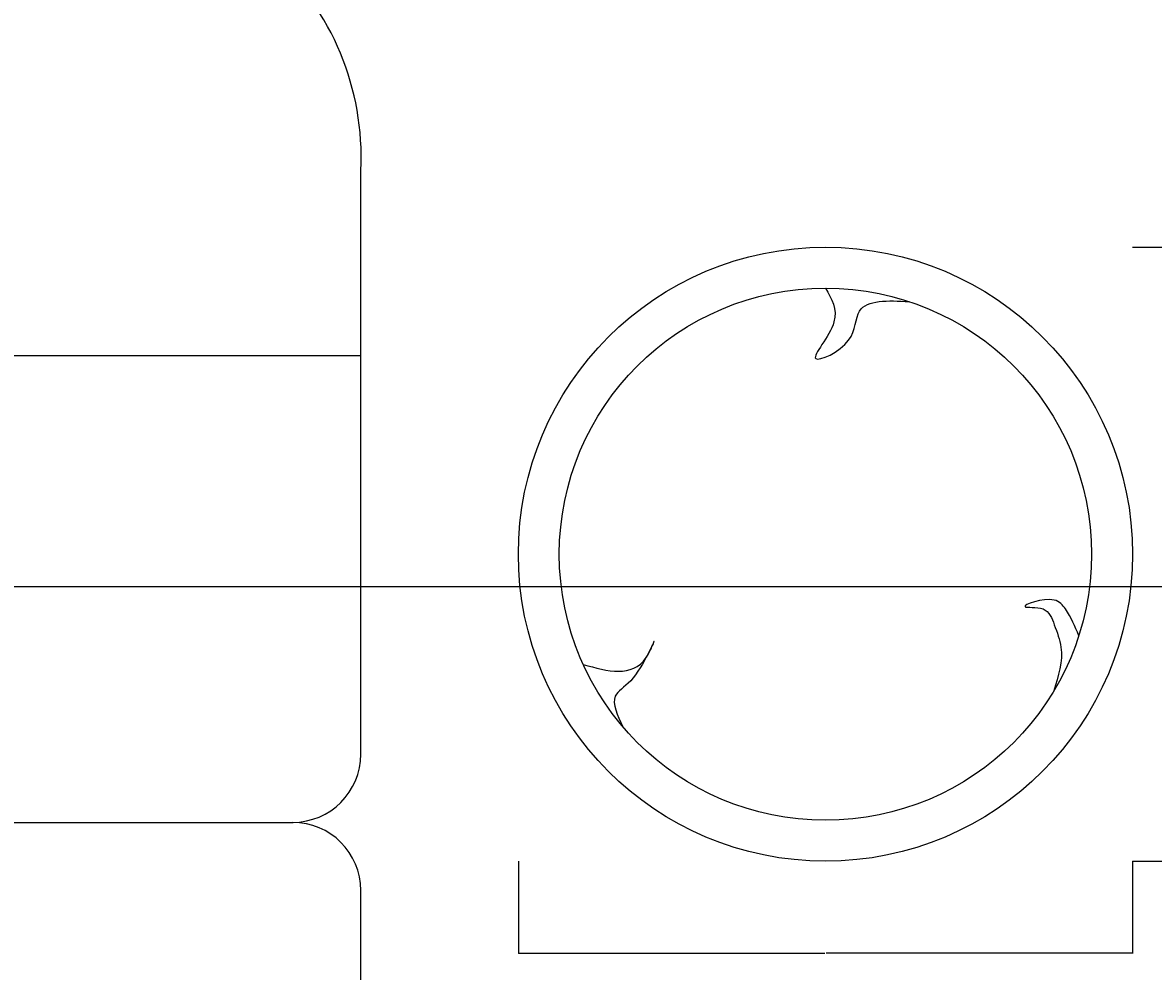
# Model space of a CAD drawing. Units: millimetres. Extents: x 19292 to 100733, y 12374 to 26974.
# Tile 12 of 24: x 28279 to 29777, y 15938 to 17195. Entities that reach past the tile are written whole.
import ezdxf

# ---------------------------------------------------------------- set-up
doc = ezdxf.new("R2010")
doc.units = ezdxf.units.MM
for name, color, linetype, lineweight in [('A-ANNO-DIMS', 2, 'Continuous', 18), ('A-FLOR-PATT', 252, 'Continuous', 13), ('A-FURN', 8, 'Continuous', 18)]:
    doc.layers.add(name, color=color, linetype=linetype, lineweight=lineweight)
doc.layers.add('FURNITURE', color=40, linetype='Continuous')
doc.styles.get("Standard").update_dxf_attribs({"font": 'arial.ttf'})
doc.dimstyles.get("Standard").update_dxf_attribs({"dimtxt": 0.18, "dimasz": 0.18, "dimexe": 0.18, "dimexo": 0.0625, "dimgap": 0.09, "dimtad": 0, "dimtih": 1, "dimtoh": 1, "dimdec": 4, "dimzin": 0, "dimdsep": 46, "dimtxsty": 'Standard', "dimcen": 0.09, "dimadec": 0, "dimazin": 0, "dimtfac": 1, "dimtdec": 4, "dimtofl": 0, "dimtmove": 0, "dimatfit": 3, "dimfxl": 1, "dimtolj": 1, "dimtzin": 0, "dimarcsym": 0})

# ---------------------------------------------------------------- blocks, each defined once
blk = doc.blocks.new('2sofa-hf')
at = {"layer": 'FURNITURE'}
for p, q in [((-27, -29.849), (-27, 31.724)), ((-21.6, -24.449), (-21.6, 31.724)), ((-21.6, 31.724), (-13.688, 31.724)), ((0, -6.325), (0, 19.345)), ((-21.616, 11.2), (-0.016, 11.2)), ((-21.573, -9.325), (-2.973, -9.325)), ((0, -23.849), (0, -12.325)), ((-16.2, -29.849), (-3, -29.849)), ((-21.6, -35.249), (-2.43, -35.249))]:
    blk.add_line(p, q, dxfattribs=at)
for centre, radius, start, end in [((-24.3, 32.033), 2.718, 353.479, 186.521), ((-11.919, 19.923), 11.933, 357.2261, 98.5207), ((-3, -6.325), 3, 270, 0), ((-3, -12.325), 3, 0, 90), ((-6, -23.849), 6, 270, 0), ((-16.2, -24.449), 5.4, 180, 270), ((-21.6, -29.849), 5.4, 180, 270), ((-2.715, -32.549), 2.715, 263.9744, 96.0256)]:
    blk.add_arc(centre, radius, start, end, dxfattribs=at)
blk = doc.blocks.new('PUFFY')
at = {"layer": 'FURNITURE', "const_width": 0.00005}
for points in [[(-0.429, 6.161, 1), (-0.417, 6.161, 1)], [(-1.711, 5.906, 1), (-1.698, 5.906, 1)], [(-1.249, 6.008, 1), (-1.237, 6.008, 1)], [(-0.276, 5.803, 1), (-0.263, 5.803, 1)], [(1.262, 5.803, 1), (1.274, 5.803, 1)], [(1.877, 5.547, 1), (1.889, 5.547, 1)], [(2.697, 5.547, 1), (2.709, 5.547, 1)], [(-2.479, 5.496, 1), (-2.467, 5.496, 1)], [(-1.916, 5.394, 1), (-1.903, 5.394, 1)], [(-0.891, 5.496, 1), (-0.878, 5.496, 1)], [(1.415, 5.343, 1), (1.428, 5.343, 1)], [(-2.787, 5.138, 1), (-2.774, 5.138, 1)], [(-2.428, 5.036, 1), (-2.416, 5.036, 1)], [(-1.864, 5.036, 1), (-1.852, 5.036, 1)], [(-1.147, 5.036, 1), (-1.134, 5.036, 1)], [(0.8, 5.036, 1), (0.813, 5.036, 1)], [(1.569, 4.933, 1), (1.582, 4.933, 1)], [(2.184, 4.882, 1), (2.197, 4.882, 1)], [(2.85, 4.933, 1), (2.863, 4.933, 1)], [(-2.479, 4.524, 1), (-2.467, 4.524, 1)], [(-1.659, 4.575, 1), (-1.647, 4.575, 1)], [(-0.686, 4.626, 1), (-0.673, 4.626, 1)], [(1.569, 4.421, 1), (1.582, 4.421, 1)], [(-1.198, 4.37, 1), (-1.186, 4.37, 1)], [(1.159, 4.319, 1), (1.172, 4.319, 1)], [(2.44, 4.268, 1), (2.453, 4.268, 1)], [(3.824, -1.464, 1), (3.837, -1.464, 1)], [(4.593, -1.822, 1), (4.606, -1.822, 1)], [(4.029, -2.129, 1), (4.042, -2.129, 1)], [(5.054, -2.026, 1), (5.067, -2.026, 1)], [(4.542, -2.231, 1), (4.554, -2.231, 1)], [(5.105, -2.487, 1), (5.118, -2.487, 1)], [(3.722, -2.538, 1), (3.734, -2.538, 1)], [(4.439, -2.692, 1), (4.452, -2.692, 1)], [(-3.453, -2.896, 1), (-3.441, -2.896, 1)], [(4.183, -2.896, 1), (4.196, -2.896, 1)], [(-4.581, -3.306, 1), (-4.568, -3.306, 1)], [(-4.068, -3.306, 1), (-4.056, -3.306, 1)], [(3.619, -3.05, 1), (3.632, -3.05, 1)], [(4.9, -3.05, 1), (4.913, -3.05, 1)], [(5.31, -3.204, 1), (5.323, -3.204, 1)], [(-3.094, -3.459, 1), (-3.082, -3.459, 1)], [(3.875, -3.562, 1), (3.888, -3.562, 1)], [(4.49, -3.459, 1), (4.503, -3.459, 1)], [(-4.786, -3.818, 1), (-4.773, -3.818, 1)], [(-3.709, -3.766, 1), (-3.697, -3.766, 1)], [(5.157, -3.664, 1), (5.169, -3.664, 1)], [(-4.222, -3.92, 1), (-4.209, -3.92, 1)], [(-3.197, -4.073, 1), (-3.184, -4.073, 1)], [(4.49, -3.971, 1), (4.503, -3.971, 1)], [(-3.914, -4.227, 1), (-3.902, -4.227, 1)], [(3.67, -4.329, 1), (3.683, -4.329, 1)], [(4.132, -4.278, 1), (4.144, -4.278, 1)], [(-4.324, -4.483, 1), (-4.312, -4.483, 1)], [(-3.453, -4.483, 1), (-3.441, -4.483, 1)], [(-2.736, -4.483, 1), (-2.723, -4.483, 1)], [(-3.812, -4.892, 1), (-3.799, -4.892, 1)], [(-3.146, -5.046, 1), (-3.133, -5.046, 1)], [(-2.531, -5.353, 1), (-2.518, -5.353, 1)]]:
    blk.add_lwpolyline(points, format="xyb", close=True, dxfattribs=at)
at = {"layer": 'FURNITURE'}
for radius in [7.5, 6.5]:
    blk.add_circle((0, 0), radius, dxfattribs=at)
for points, knots in [([(0, 6.5), (0.148, 6.243), (0.47, 5.685), (-0.715, 4.457), (0.771, 5.119), (0.69, 6.238), (1.526, 6.197), (2.042, 6.171)], [0, 0, 0, 0, 0.853207, 1.850764, 2.77014, 3.532386, 4.762324, 4.762324, 4.762324, 4.762324]), ([(6.187, -1.993), (6.093, -1.767), (5.955, -1.431), (5.557, -0.962), (4.503, -1.357), (5.424, -1.248), (5.598, -1.766), (5.859, -2.423), (5.689, -2.977), (5.577, -3.339)], [0, 0, 0, 0, 0.731037, 1.082325, 1.814636, 2.257188, 2.72894, 3.301273, 4.384204, 4.384204, 4.384204, 4.384204]), ([(-5.915, -2.694), (-5.318, -2.862), (-4.56, -3.069), (-4.022, -1.724), (-4.58, -3.096), (-5.312, -3.455), (-5.082, -3.934), (-4.946, -4.218)], [0.010289, 0.010289, 0.010289, 0.010289, 1.160744, 1.473738, 2.290002, 2.686083, 3.263094, 3.263094, 3.263094, 3.263094])]:
    blk.add_open_spline(points, degree=3, knots=knots, dxfattribs=at)
blk = doc.blocks.new('*D46')
at = {"layer": 'A-ANNO-DIMS', "color": 0, "lineweight": -2, "transparency": 16777216}
for p, q in [((28935.4, 16083.8), (28935.4, 15961.6)), ((29749.1, 16083.8), (29749.1, 15961.6)), ((28935.6, 15961.8), (29341.3, 15961.8)), ((29748.9, 15961.8), (29343.2, 15961.8))]:
    blk.add_line(p, q, dxfattribs=at)
at = {"layer": 'A-ANNO-DIMS', "color": 0, "transparency": 16777216}
for points in [[(28935.6, 15961.8), (28935.6, 15961.7), (28935.4, 15961.8)], [(29748.9, 15961.8), (29748.9, 15961.7), (29749.1, 15961.8)]]:
    blk.add_solid(points, dxfattribs=at)
at = {"layer": 'Defpoints', "color": 0, "transparency": 16777216}
for p in [(28935.4, 16083.8), (29749.1, 16083.8), (29749.1, 15961.8)]:
    blk.add_point(p, dxfattribs=at)
at = {"layer": 'A-ANNO-DIMS', "color": 0, "transparency": 16777216, "insert": (29342.3, 15961.8), "char_height": 0.18, "attachment_point": 5}
blk.add_mtext('\\A1;POUF 814 TYP.', dxfattribs=at)
blk = doc.blocks.new('*D47')
at = {"layer": 'A-ANNO-DIMS', "color": 0, "lineweight": -2, "transparency": 16777216}
for p, q in [((29749.2, 16897.5), (29871.3, 16897.5)), ((29871.2, 16897.4), (29871.2, 16490.9)), ((29871.2, 16084), (29871.2, 16490.5)), ((29749.2, 16083.8), (29871.3, 16083.8))]:
    blk.add_line(p, q, dxfattribs=at)
at = {"layer": 'A-ANNO-DIMS', "color": 0, "transparency": 16777216}
for points in [[(29871.1, 16897.4), (29871.2, 16897.4), (29871.2, 16897.5)], [(29871.1, 16084), (29871.2, 16084), (29871.2, 16083.8)]]:
    blk.add_solid(points, dxfattribs=at)
at = {"layer": 'Defpoints', "color": 0, "transparency": 16777216}
for p in [(29749.1, 16897.5), (29871.2, 16897.5), (29749.1, 16083.8)]:
    blk.add_point(p, dxfattribs=at)
at = {"layer": 'A-ANNO-DIMS', "color": 0, "transparency": 16777216, "insert": (29871.2, 16490.7), "char_height": 0.18, "attachment_point": 5}
blk.add_mtext('\\A1;814 TYP.', dxfattribs=at)
blk = doc.blocks.new('*D70')
at = {"layer": 'A-ANNO-DIMS', "color": 0, "lineweight": -2, "transparency": 16777216}
for p, q in [((23573.9, 17387.7), (36879.3, 17387.7)), ((36879.2, 17387.6), (36879.2, 16917.9)), ((36879.2, 16447.9), (36879.2, 16917.6)), ((23573.9, 16447.7), (36879.3, 16447.7))]:
    blk.add_line(p, q, dxfattribs=at)
at = {"layer": 'A-ANNO-DIMS', "color": 0, "transparency": 16777216}
for points in [[(36879.1, 17387.6), (36879.2, 17387.6), (36879.2, 17387.7)], [(36879.1, 16447.9), (36879.2, 16447.9), (36879.2, 16447.7)]]:
    blk.add_solid(points, dxfattribs=at)
at = {"layer": 'Defpoints', "color": 0, "transparency": 16777216}
for p in [(23573.8, 17387.7), (36879.2, 17387.7), (23573.8, 16447.7)]:
    blk.add_point(p, dxfattribs=at)
at = {"layer": 'A-ANNO-DIMS', "color": 0, "transparency": 16777216, "insert": (36879.2, 16917.7), "char_height": 0.18, "attachment_point": 5}
blk.add_mtext('\\A1;940', dxfattribs=at)
blk = doc.blocks.new('*D79')
at = {"layer": 'A-ANNO-DIMS', "color": 0, "lineweight": -2, "transparency": 16777216}
for p, q in [((22694.1, 22860.7), (22694.1, 12808.8)), ((36144.2, 15985.7), (36144.2, 12808.8)), ((22694.3, 12809), (29418.7, 12809)), ((36144, 12809), (29419.6, 12809))]:
    blk.add_line(p, q, dxfattribs=at)
at = {"layer": 'A-ANNO-DIMS', "color": 0, "transparency": 16777216}
for points in [[(22694.3, 12809), (22694.3, 12809), (22694.1, 12809)], [(36144, 12809), (36144, 12809), (36144.2, 12809)]]:
    blk.add_solid(points, dxfattribs=at)
at = {"layer": 'Defpoints', "color": 0, "transparency": 16777216}
for p in [(22694.1, 22860.7), (36144.2, 15985.7), (36144.2, 12809)]:
    blk.add_point(p, dxfattribs=at)
at = {"layer": 'A-ANNO-DIMS', "color": 0, "transparency": 16777216, "insert": (29419.2, 12809), "char_height": 0.18, "attachment_point": 5}
blk.add_mtext('\\A1;13450', dxfattribs=at)
blk = doc.blocks.new('*D82')
at = {"layer": 'A-ANNO-DIMS', "color": 0, "lineweight": -2, "transparency": 16777216}
for p, q in [((27198.8, 13562.8), (27198.8, 23555.9)), ((27199, 23555.7), (29296.4, 23555.7)), ((31394.6, 23555.7), (29297.2, 23555.7)), ((31394.8, 13544.1), (31394.8, 23555.9))]:
    blk.add_line(p, q, dxfattribs=at)
at = {"layer": 'A-ANNO-DIMS', "color": 0, "transparency": 16777216}
for points in [[(27199, 23555.8), (27199, 23555.7), (27198.8, 23555.7)], [(31394.6, 23555.8), (31394.6, 23555.7), (31394.8, 23555.7)]]:
    blk.add_solid(points, dxfattribs=at)
at = {"layer": 'Defpoints', "color": 0, "transparency": 16777216}
for p in [(31394.8, 23555.7), (27198.8, 13562.7), (31394.8, 13544)]:
    blk.add_point(p, dxfattribs=at)
at = {"layer": 'A-ANNO-DIMS', "color": 0, "transparency": 16777216, "insert": (29296.8, 23555.7), "char_height": 0.18, "attachment_point": 5}
blk.add_mtext('\\A1;4196', dxfattribs=at)
blk = doc.blocks.new('*D86')
at = {"layer": 'A-ANNO-DIMS', "color": 0, "lineweight": -2, "transparency": 16777216}
for p, q in [((27198.8, 15132.8), (27198.8, 23555.9)), ((27199, 23555.7), (29198.5, 23555.7)), ((31198.6, 23555.7), (29199.2, 23555.7)), ((31198.8, 15132.8), (31198.8, 23555.9))]:
    blk.add_line(p, q, dxfattribs=at)
at = {"layer": 'A-ANNO-DIMS', "color": 0, "transparency": 16777216}
for points in [[(27199, 23555.8), (27199, 23555.7), (27198.8, 23555.7)], [(31198.6, 23555.8), (31198.6, 23555.7), (31198.8, 23555.7)]]:
    blk.add_solid(points, dxfattribs=at)
at = {"layer": 'Defpoints', "color": 0, "transparency": 16777216}
for p in [(31198.8, 23555.7), (27198.8, 15132.7), (31198.8, 15132.7)]:
    blk.add_point(p, dxfattribs=at)
at = {"layer": 'A-ANNO-DIMS', "color": 0, "transparency": 16777216, "insert": (29198.8, 23555.7), "char_height": 0.18, "attachment_point": 5}
blk.add_mtext('\\A1;4000', dxfattribs=at)

msp = doc.modelspace()

# ---------------------------------------------------------------- hatches: boundary and pattern name
at = {"layer": 'A-FLOR-PATT'}
h = msp.add_hatch(dxfattribs=at)
h.set_pattern_fill('CROSS', color=256, scale=40)
h.paths.add_polyline_path([(36144.169, 19010.725), (33719.169, 19010.725), (33719.169, 18850.725), (33719.169, 18003.026), (33719.169, 15985.725), (36144.169, 15985.725)])
h.paths.add_polyline_path([(36144.132, 22460.725), (34419.132, 22460.725), (34419.132, 22208.026, -0.34415073), (35121.831, 21308.026), (34419.132, 21308.026), (34419.132, 21260.725), (36144.132, 21260.725)])
h.paths.add_polyline_path([(34419.132, 22208.026), (34419.132, 21388.026), (35118.375, 21388.026, 0.32018294)], flags=17)
h.paths.add_polyline_path([(31169.132, 22460.725), (28369.132, 22460.725), (28369.132, 21460.725), (31169.132, 21460.725)])
h.paths.add_polyline_path([(34010.406, 17316.149), (36018.156, 17316.149), (36018.156, 17722.778), (34010.406, 17722.778)], flags=24)
h.paths.add_polyline_path([(34456.896, 21920.301), (35605.434, 21920.301), (35605.434, 22313.518), (34456.896, 22313.518)], flags=25)
h.paths.add_polyline_path([(29263.068, 21823.707), (30421.489, 21823.707), (30421.489, 22034.008), (29263.068, 22034.008)], flags=24)

# ---------------------------------------------------------------- block references
at = {"layer": 'A-FURN'}
for name, p, xscale, yscale, zscale in [('2sofa-hf', (28726.739, 16416.302), 30.13269765108242, 30.13269765108242, 30.13269765108242), ('PUFFY', (29342.259, 16490.677), 54.24717212198793, 54.24717212198793, 54.24717212198793)]:
    msp.add_blockref(name, p, dxfattribs=dict(at, xscale=xscale, yscale=yscale, zscale=zscale))

# ---------------------------------------------------------------- dimensions: what is measured, and where the dimension line sits
at = {"layer": 'A-ANNO-DIMS'}
for base, p1, p2, picture, middle in [((31394.799, 23555.725), (27198.815, 13562.748), (31394.799, 13543.993), '*D82', (29296.807, 23555.725)), ((31198.815, 23555.725), (27198.815, 15132.748), (31198.815, 15132.748), '*D86', (29198.815, 23555.725)), ((36144.169, 12808.993), (22694.132, 22860.725), (36144.169, 15985.725), '*D79', (29419.151, 12808.993))]:
    dim = msp.add_linear_dim(base=base, p1=p1, p2=p2, dimstyle='Standard', override={"dimdec": 0, "dimlfac": 1, "dimrnd": 0, "dimzin": 0, "dimdsep": 46, "dimlunit": 2}, dxfattribs=at)
    dim.commit()
    dim.dimension.update_dxf_attribs({"geometry": picture, "text_midpoint": middle})
dim = msp.add_linear_dim(base=(36879.169, 17387.748), p1=(23573.815, 16447.748), p2=(23573.815, 17387.748), angle=90, dimstyle='Standard', override={"dimdec": 0, "dimlfac": 1, "dimrnd": 0, "dimzin": 0, "dimdsep": 46, "dimlunit": 2}, dxfattribs=at)
dim.commit()
dim.dimension.update_dxf_attribs({"geometry": '*D70', "text_midpoint": (36879.169, 16917.748)})
dim = msp.add_linear_dim(base=(29871.169, 16897.53), p1=(29749.113, 16083.823), p2=(29749.113, 16897.53), angle=90, text='<> TYP.', dimstyle='Standard', override={"dimdec": 0, "dimrnd": 0, "dimzin": 0, "dimlunit": 2}, dxfattribs=at)
dim.commit()
dim.dimension.update_dxf_attribs({"geometry": '*D47', "text_midpoint": (29871.169, 16490.677)})
dim = msp.add_linear_dim(base=(29749.113, 15961.767), p1=(28935.405, 16083.823), p2=(29749.113, 16083.823), text='POUF <> TYP.', dimstyle='Standard', override={"dimdec": 0, "dimrnd": 0, "dimzin": 0, "dimlunit": 2}, dxfattribs=at)
dim.commit()
dim.dimension.update_dxf_attribs({"geometry": '*D46', "text_midpoint": (29342.259, 15961.767)})

doc.saveas('drawing.dxf')
